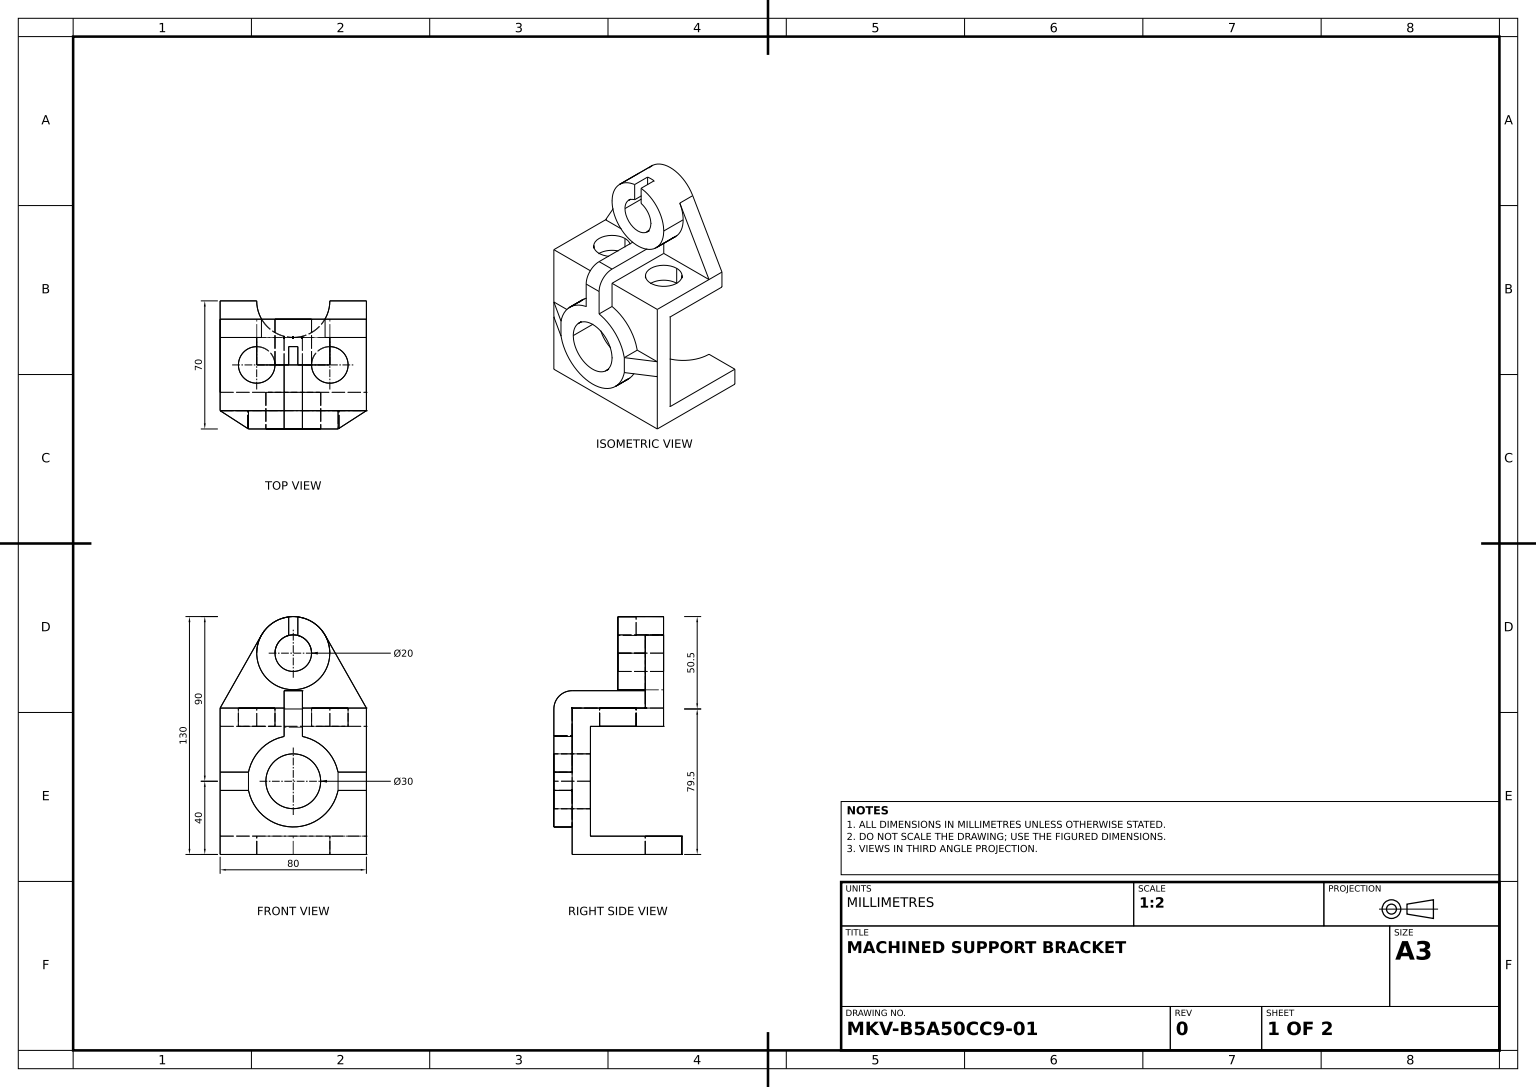
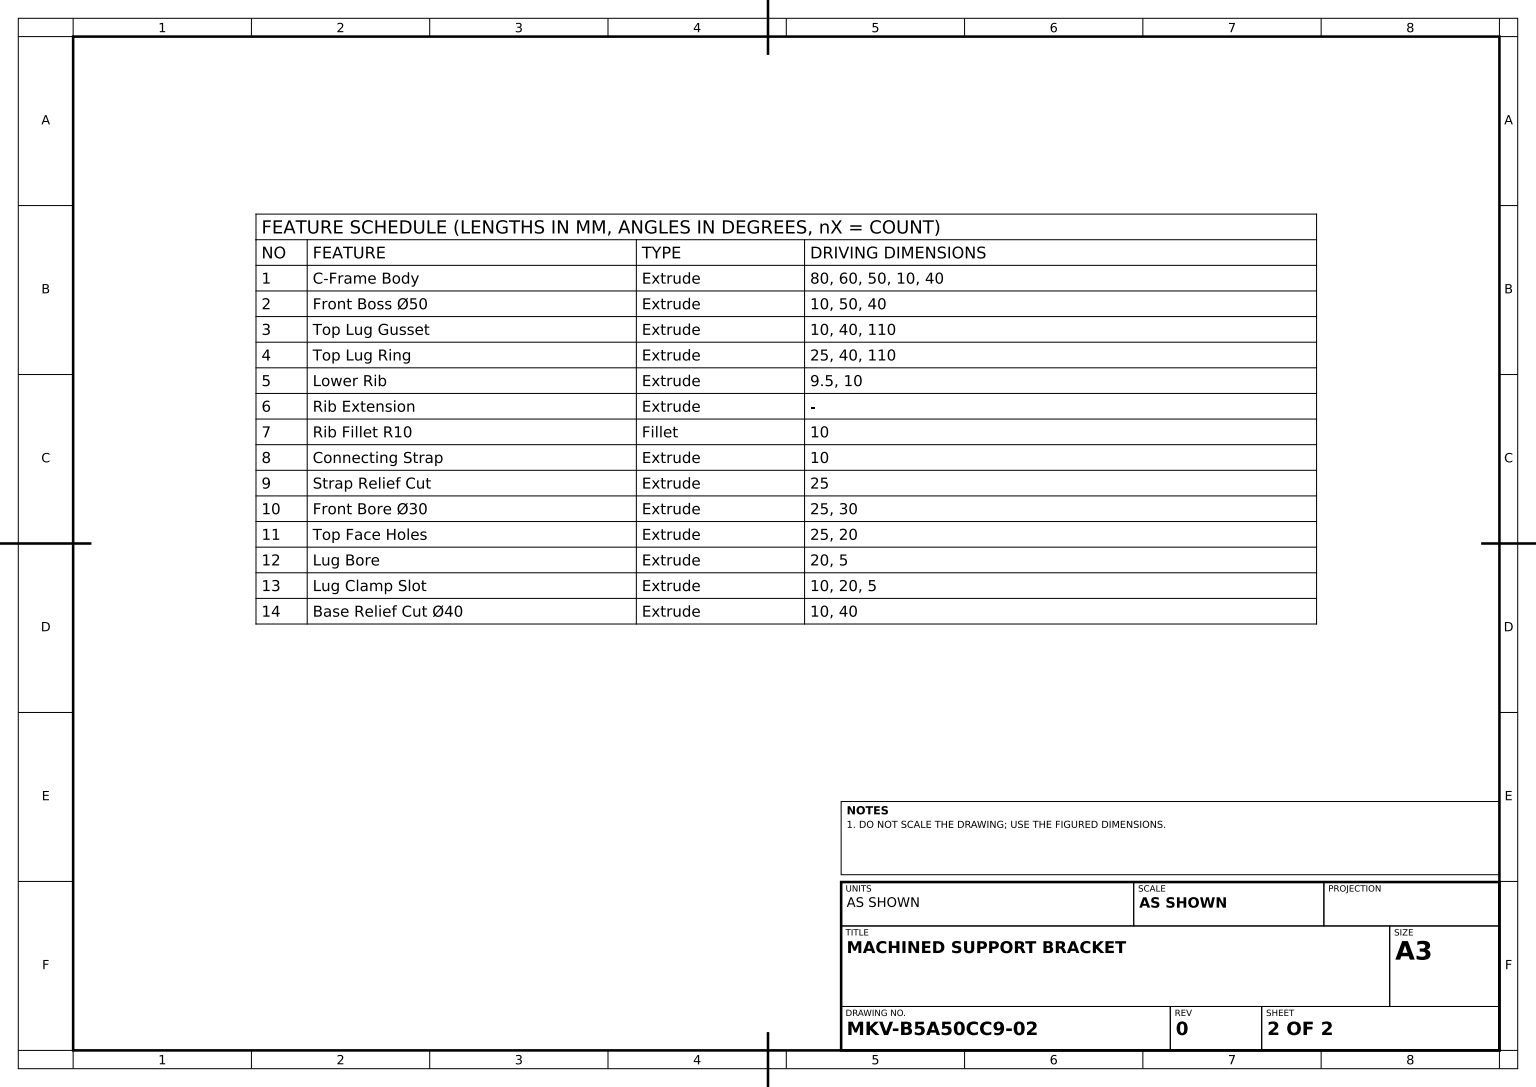
from build123d import *

# Parameters (mm, degrees)
C_FRAME_BODY_DEPTH        = 80
FRONT_BOSS_SKETCH_R       = 25
FRONT_BOSS_50_DEPTH       = 10
TOP_LUG_GUSSET_DEPTH      = 10
SKETCH3_3_R               = 20
TOP_LUG_RING_DEPTH        = 25
LOWER_RIB_REACH           = 169.929
LOWER_RIB_SKETCH_W        = 10
LOWER_RIB_SKETCH_H        = 9.5
RIB_EXTENSION_REACH       = 135.041
RIB_EXTENSION_SKETCH_W    = 10
RIB_EXTENSION_SKETCH_H    = 10
RIB_FILLET_R10_R          = 10
CONNECTING_STRAP_REACH    = 169.929
CONNECTING_STRAP_SKETCH_W = 15.505102572
CONNECTING_STRAP_SKETCH_H = 10
STRAP_RELIEF_CUT_DEPTH    = 25
FRONT_BORE_SKETCH_R       = 15
FRONT_BORE_30_DEPTH       = 25
TOP_HOLES_SKETCH_R        = 10
TOP_FACE_HOLES_DEPTH      = 25
LUG_BORE_DEPTH            = 157.604597634
LUG_CLAMP_SLOT_DEPTH      = 10
BASE_RELIEF_SKETCH_R      = 20
BASE_RELIEF_CUT_40_DEPTH  = 10


with BuildPart() as part:
    # C-Frame Profile Sketch → C-Frame Body (new body)
    with BuildSketch(Plane(origin=(0, 0, 0), x_dir=(0, 0, -1), z_dir=(1, 0, 0))):
        Polygon((0, 0), (-60, 0), (-60, 80), (-10, 80), (-10, 70), (-50, 70), (-50, 10), (0, 10), align=None)
    extrude(amount=-C_FRAME_BODY_DEPTH)

    # Front Boss Sketch → Front Boss _50 (add)
    with BuildSketch(Plane.XY.offset(60)):
        with Locations((-40, 40)):
            Circle(FRONT_BOSS_SKETCH_R)
    extrude(amount=FRONT_BOSS_50_DEPTH)

    # Top Lug Sketch → Top Lug Gusset (add)
    with BuildSketch(Plane(origin=(0, 0, 10), x_dir=(-1, 0, 0), z_dir=(0, 0, -1))):
        with BuildLine():
            ThreePointArc((60, 110), (34.899197777, 90.661390518), (22.601818332, 119.864242224))
            Line((22.601818332, 119.864242224), (0, 80))
            Line((0, 80), (80, 80))
            Line((80, 80), (57.398181668, 119.864242224))
            ThreePointArc((57.398181668, 119.864242224), (59.338609482, 115.100802223), (60, 110))
        make_face()
    extrude(amount=-TOP_LUG_GUSSET_DEPTH)

    # Sketch3_3 → Top Lug Ring (add)
    with BuildSketch(Plane(origin=(0, 0, 10), x_dir=(-1, 0, 0), z_dir=(0, 0, -1))):
        with Locations((40, 110)):
            Circle(SKETCH3_3_R)
    extrude(amount=-TOP_LUG_RING_DEPTH)

    # Lower Rib Sketch → Lower Rib (add, up to next)
    with BuildSketch(Plane.XY.offset(70), mode=Mode.PRIVATE) as lower_rib_sk1:
        with Locations((-40, 84.75)):
            Rectangle(LOWER_RIB_SKETCH_W, LOWER_RIB_SKETCH_H)
    lower_rib_tool1 = extrude(lower_rib_sk1.sketch, amount=-LOWER_RIB_REACH, mode=Mode.PRIVATE) - part.part
    add(lower_rib_tool1.solids().sort_by_distance((-40, 84.75, 70))[0])

    # Rib Extension Sketch → Rib Extension (add, up to next)
    with BuildSketch(Plane.XZ.offset(-80), mode=Mode.PRIVATE) as rib_extension_sk1:
        with Locations((-40, 65)):
            Rectangle(RIB_EXTENSION_SKETCH_W, RIB_EXTENSION_SKETCH_H)
    rib_extension_tool1 = extrude(rib_extension_sk1.sketch, amount=RIB_EXTENSION_REACH, mode=Mode.PRIVATE) - part.part
    add(rib_extension_tool1.solids().sort_by_distance((-40, 80, 65))[0])

    # Rib Fillet R10
    rib_fillet_r10_edges = [part.edges().sort_by_distance(p)[0] for p in [
        (-40, 89.5, 70),
    ]]
    fillet(rib_fillet_r10_edges, radius=RIB_FILLET_R10_R)

    # Connecting Strap Sketch → Connecting Strap (add, up to next)
    with BuildSketch(Plane.XY.offset(70), mode=Mode.PRIVATE) as connecting_strap_sk1:
        with Locations((-7.752551286, 40)):
            Rectangle(CONNECTING_STRAP_SKETCH_W, CONNECTING_STRAP_SKETCH_H)
    connecting_strap_tool1 = extrude(connecting_strap_sk1.sketch, amount=-CONNECTING_STRAP_REACH, mode=Mode.PRIVATE) - part.part
    # Connecting Strap Sketch → Connecting Strap (add, up to next)
    with BuildSketch(Plane.XY.offset(70), mode=Mode.PRIVATE) as connecting_strap_sk2:
        with Locations((-72.247448714, 40)):
            Rectangle(CONNECTING_STRAP_SKETCH_W, CONNECTING_STRAP_SKETCH_H)
    connecting_strap_tool2 = extrude(connecting_strap_sk2.sketch, amount=-CONNECTING_STRAP_REACH, mode=Mode.PRIVATE) - part.part
    add(connecting_strap_tool1.solids().sort_by_distance((-7.752551, 40, 70))[0])
    add(connecting_strap_tool2.solids().sort_by_distance((-72.247449, 40, 70))[0])

    # Strap Relief Sketch → Strap Relief Cut (cut)
    with BuildSketch(Plane(origin=(0, 45, 0), x_dir=(1, 0, 0), z_dir=(0, 1, 0))):
        Polygon((-15.505102572, -70), (0, -60), (0, -70), align=None)
        Polygon((-80, -60), (-64.494897428, -70), (-80, -70), align=None)
    extrude(amount=-STRAP_RELIEF_CUT_DEPTH, mode=Mode.SUBTRACT)

    # Front Bore Sketch → Front Bore _30 (cut)
    with BuildSketch(Plane.XY.offset(70)):
        with Locations((-40, 40)):
            Circle(FRONT_BORE_SKETCH_R)
    extrude(amount=-FRONT_BORE_30_DEPTH, mode=Mode.SUBTRACT)

    # Top Holes Sketch → Top Face Holes (cut)
    with BuildSketch(Plane(origin=(0, 80, 0), x_dir=(1, 0, 0), z_dir=(0, 1, 0))):
        with Locations(Location((-20, -35, 0), (0, 0, 270))):
            Circle(TOP_HOLES_SKETCH_R)
        with Locations(Location((-60, -35, 0), (0, 0, 270))):
            Circle(TOP_HOLES_SKETCH_R)
    extrude(amount=-TOP_FACE_HOLES_DEPTH, mode=Mode.SUBTRACT)

    # Lug Bore and Slot Sketch → Lug Bore (cut, through all)
    with BuildSketch(Plane.XY.offset(35)):
        with BuildLine():
            ThreePointArc((-37.5, 119.682458366), (-40, 120), (-42.5, 119.682458366))
            Line((-42.5, 119.682458366), (-37.5, 119.682458366))
        make_face()
        with BuildLine():
            Line((-37.5, 119.682458366), (-42.5, 119.682458366))
            ThreePointArc((-42.5, 119.682458366), (-46.123724357, 102.09430585), (-30, 110))
            ThreePointArc((-30, 110), (-32.09430585, 116.123724357), (-37.5, 119.682458366))
        make_face()
        with BuildLine():
            ThreePointArc((-37.5, 119.682458366), (-40, 120), (-42.5, 119.682458366))
            Line((-42.5, 119.682458366), (-37.5, 119.682458366))
        make_face()
        with BuildLine():
            Line((-37.5, 119.682458366), (-42.5, 119.682458366))
            ThreePointArc((-42.5, 119.682458366), (-46.123724357, 102.09430585), (-30, 110))
            ThreePointArc((-30, 110), (-32.09430585, 116.123724357), (-37.5, 119.682458366))
        make_face()
    extrude(amount=-LUG_BORE_DEPTH, mode=Mode.SUBTRACT)

    # Sketch14_3 → Lug Clamp Slot (cut)
    with BuildSketch(Plane.XY.offset(35)):
        with BuildLine():
            Line((-42.5, 129.843134833), (-42.5, 119.682458366))
            ThreePointArc((-42.5, 119.682458366), (-40, 120), (-37.5, 119.682458366))
            Line((-37.5, 119.682458366), (-37.5, 129.843134833))
            ThreePointArc((-37.5, 129.843134833), (-40, 130), (-42.5, 129.843134833))
        make_face()
    extrude(amount=-LUG_CLAMP_SLOT_DEPTH, mode=Mode.SUBTRACT)

    # Base Relief Sketch → Base Relief Cut _40 (cut)
    with BuildSketch(Plane(origin=(0, 10, 0), x_dir=(1, 0, 0), z_dir=(0, 1, 0))):
        with Locations((-40, 0)):
            Circle(BASE_RELIEF_SKETCH_R)
    extrude(amount=-BASE_RELIEF_CUT_40_DEPTH, mode=Mode.SUBTRACT)


solid = part.part
